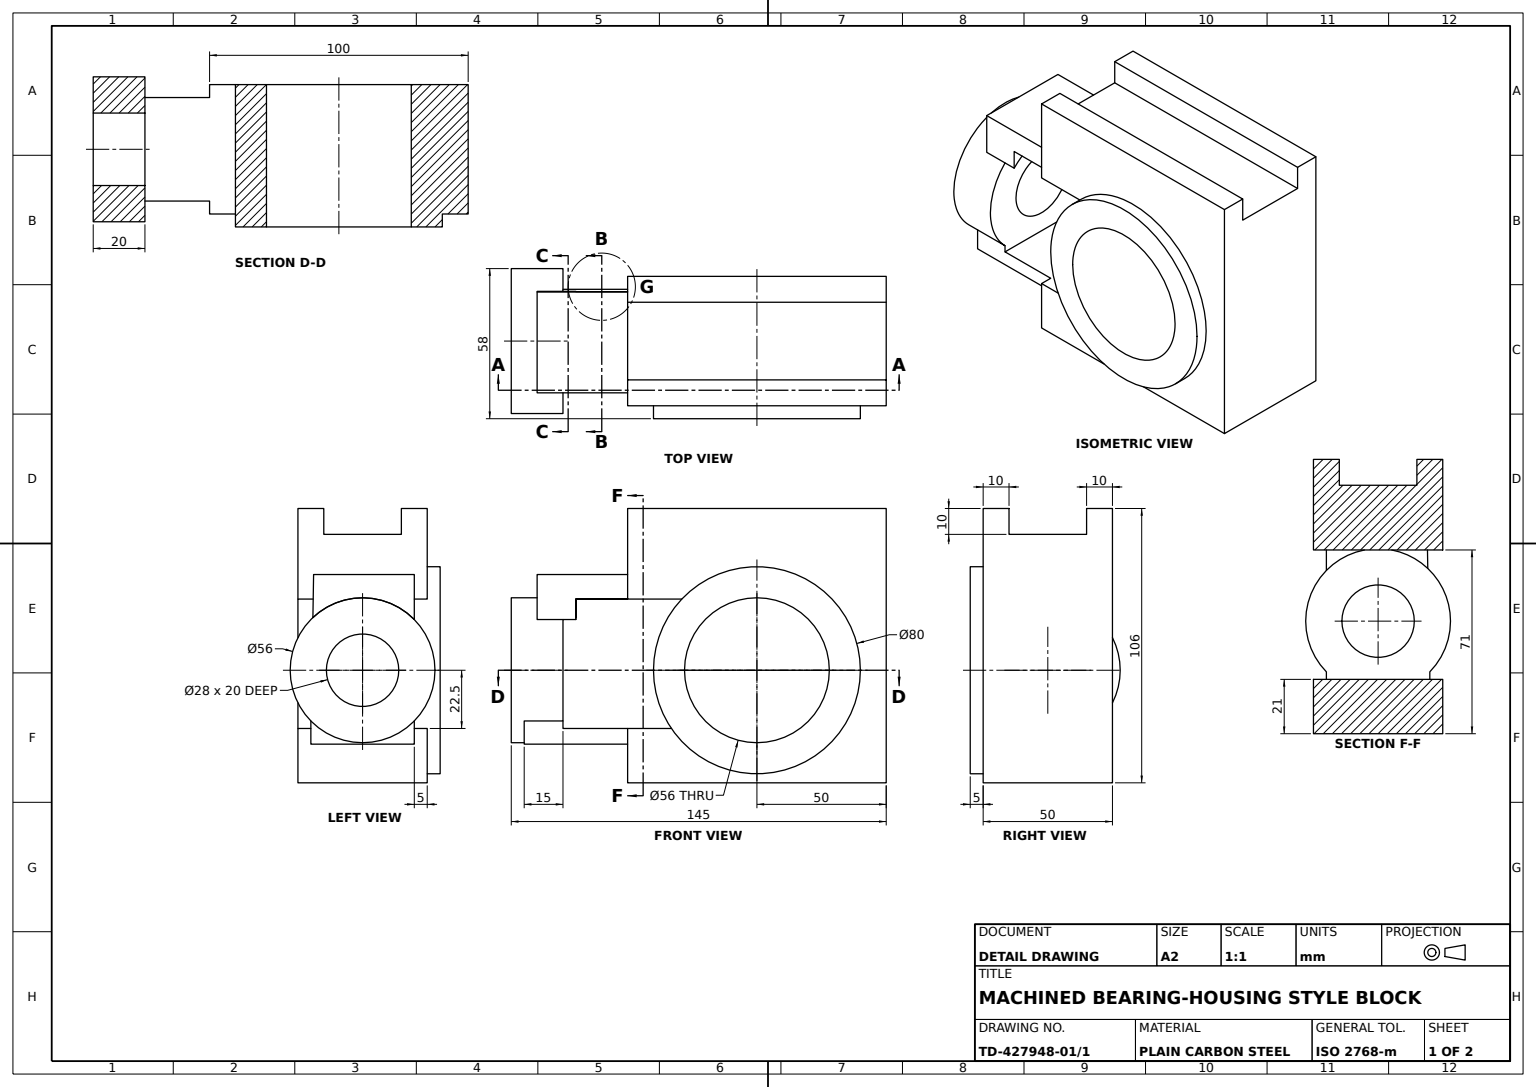
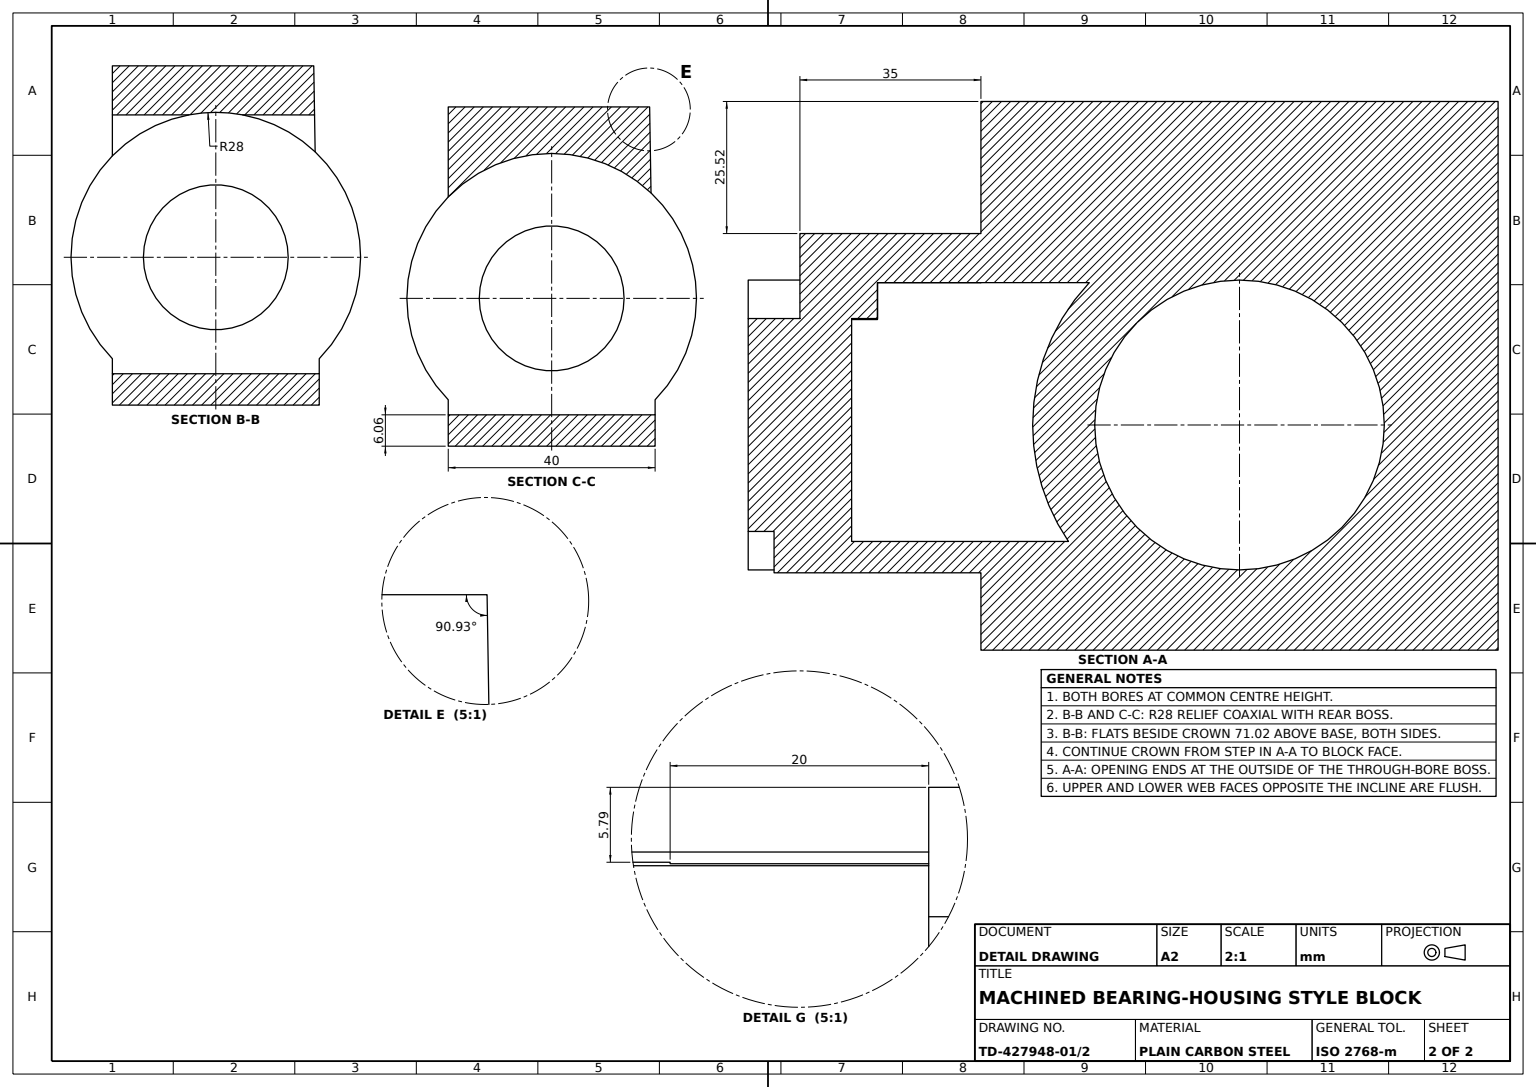
from build123d import *

# Parameters (mm, degrees)
BASE_PLATE_SKETCH_W        = 100
BASE_PLATE_SKETCH_H        = 50
BASE_PLATE_DEPTH           = 21
SIDE_WEB_SKETCH_W          = 40
SIDE_WEB_SKETCH_H          = 6.056820609
SIDE_WEB_DEPTH             = 40
REAR_BORE_BOSS_DEPTH       = 5
REAR_BORE_BOSS_DEPTH_BACK  = 15
REAR_BORE_BOSS_SKETCH_R    = 28
REAR_BORE_BOSS_SKETCH_R_2  = 14
FRONT_BORE_BOSS_DEPTH      = 5
FRONT_BORE_BOSS_DEPTH_BACK = 50
FRONT_BORE_BOSS_SKETCH_R   = 40
FRONT_BORE_BOSS_SKETCH_R_2 = 28
FRONT_BORE_REACH           = 141.145
FRONT_BORE_SKETCH_R        = 28
UPRIGHT_WALL_DEPTH         = 50
TOP_SLOT_10X10_DEPTH       = 183.101619982
TOP_SLOT_10X10_DEPTH_BACK  = 132
REAR_START                 = 35
REAR_BLOCK_DEPTH           = 35
REAR_START_2               = -20
REAR_BORE_CUT_DEPTH        = 20
REAR_LUG_DEPTH             = 15


with BuildPart() as part:
    # Base Plate Sketch → Base Plate (new body)
    with BuildSketch(Plane(origin=(0, 0, 0), x_dir=(1, 0, 0), z_dir=(0, 1, 0))):
        Rectangle(BASE_PLATE_SKETCH_W, BASE_PLATE_SKETCH_H)
    extrude(amount=BASE_PLATE_DEPTH)

    # Side Web Sketch → Side Web (add)
    with BuildSketch(Plane.ZY.offset(50)):
        with Locations((0, 17.971589696)):
            Rectangle(SIDE_WEB_SKETCH_W, SIDE_WEB_SKETCH_H)
    extrude(amount=SIDE_WEB_DEPTH)

    # Rear Bore Boss Sketch → Rear Bore Boss (add, two sides: drawn at the far end of the back side and taken through both)
    with BuildSketch(Plane.ZY.offset(90).offset(-REAR_BORE_BOSS_DEPTH_BACK)):
        with Locations((0, 43.5)):
            Circle(REAR_BORE_BOSS_SKETCH_R)
        with Locations((0, 43.5)):
            Circle(REAR_BORE_BOSS_SKETCH_R_2, mode=Mode.SUBTRACT)
    extrude(amount=REAR_BORE_BOSS_DEPTH + REAR_BORE_BOSS_DEPTH_BACK)

    # Front Bore Boss Sketch → Front Bore Boss (add, two sides: drawn at the far end of the back side and taken through both)
    with BuildSketch(Plane.XY.offset(25).offset(-FRONT_BORE_BOSS_DEPTH_BACK)):
        with Locations((0, 43.5)):
            Circle(FRONT_BORE_BOSS_SKETCH_R)
        with Locations((0, 43.5)):
            Circle(FRONT_BORE_BOSS_SKETCH_R_2, mode=Mode.SUBTRACT)
    extrude(amount=FRONT_BORE_BOSS_DEPTH + FRONT_BORE_BOSS_DEPTH_BACK)

    # Front Bore Sketch → Front Bore (cut, up to next)
    with BuildSketch(Plane.XY.offset(30), mode=Mode.PRIVATE) as front_bore_sk1:
        with Locations((0, 43.5)):
            Circle(FRONT_BORE_SKETCH_R)
    front_bore_tool1 = extrude(front_bore_sk1.sketch, amount=-FRONT_BORE_REACH, mode=Mode.PRIVATE) & part.part
    add(front_bore_tool1.solids().sort_by_distance((0, 43.5, 30))[0], mode=Mode.SUBTRACT)

    # Upright Wall Sketch → Upright Wall (add)
    with BuildSketch(Plane.XY.offset(25)):
        with BuildLine():
            Line((50, 21), (50, 106))
            Line((50, 106), (-50, 106))
            Line((-50, 106), (-50, 71))
            Line((-50, 71), (-29.047375097, 71))
            ThreePointArc((-29.047375097, 71), (25.080852913, 74.660083715), (33.071891388, 21))
            Line((33.071891388, 21), (50, 21))
        make_face()
    extrude(amount=-UPRIGHT_WALL_DEPTH)

    # Top Slot Sketch → Top Slot 10x10 (cut, two sides: drawn at the far end of the back side and taken through both)
    with BuildSketch(Plane(origin=(50, 0, 0), x_dir=(0, 0, -1), z_dir=(1, 0, 0)).offset(-TOP_SLOT_10X10_DEPTH_BACK)):
        Polygon((-15, 346.312830732), (-15, 106), (-15, 96), (15, 96), (15, 106), (15, 346.312830732), (15, 826.938492197), (-15, 826.938492197), align=None)
    extrude(amount=TOP_SLOT_10X10_DEPTH + TOP_SLOT_10X10_DEPTH_BACK, mode=Mode.SUBTRACT)

    # Rear Block Sketch → Rear Block (add)
    with BuildSketch(Plane.ZY.offset(50).offset(REAR_START)):
        with BuildLine():
            Line((-18.941471656, 80.4842707), (-19.209783437, 63.871161486))
            ThreePointArc((-19.209783437, 63.871161486), (0.553499044, 71.49452873), (20, 63.095917942))
            Line((20, 63.095917942), (20, 80.4842707))
            Line((20, 80.4842707), (-18.941471656, 80.4842707))
        make_face()
    extrude(amount=-REAR_BLOCK_DEPTH)

    # Rear Bore Cut Sketch → Rear Bore Cut (cut)
    with BuildSketch(Plane(origin=(-50, 0, 0), x_dir=(0, 0, -1), z_dir=(1, 0, 0)).offset(REAR_START_2)):
        with BuildLine():
            Line((-20, 71), (-20, 63.095917942))
            ThreePointArc((-20, 63.095917942), (-13.203990192, 68.191185532), (-5.192884853, 71.014249888))
            Line((-5.192884853, 71.014249888), (-20, 71))
        make_face()
        with BuildLine():
            Line((19.209783437, 63.871161486), (19.094648375, 71))
            Line((19.094648375, 71), (5.192884853, 71.014249888))
            ThreePointArc((5.192884853, 71.014249888), (12.713319114, 68.447374954), (19.209783437, 63.871161486))
        make_face()
    extrude(amount=REAR_BORE_CUT_DEPTH, mode=Mode.SUBTRACT)

    # Rear Lug Sketch → Rear Lug (add)
    with BuildSketch(Plane.ZY.offset(90)):
        with BuildLine():
            Line((-20, 14.943179391), (-20, 23.904082058))
            ThreePointArc((-20, 23.904082058), (0, 15.5), (20, 23.904082058))
            Line((20, 23.904082058), (20, 14.943179391))
            Line((20, 14.943179391), (-20, 14.943179391))
        make_face()
    extrude(amount=-REAR_LUG_DEPTH)


solid = part.part
